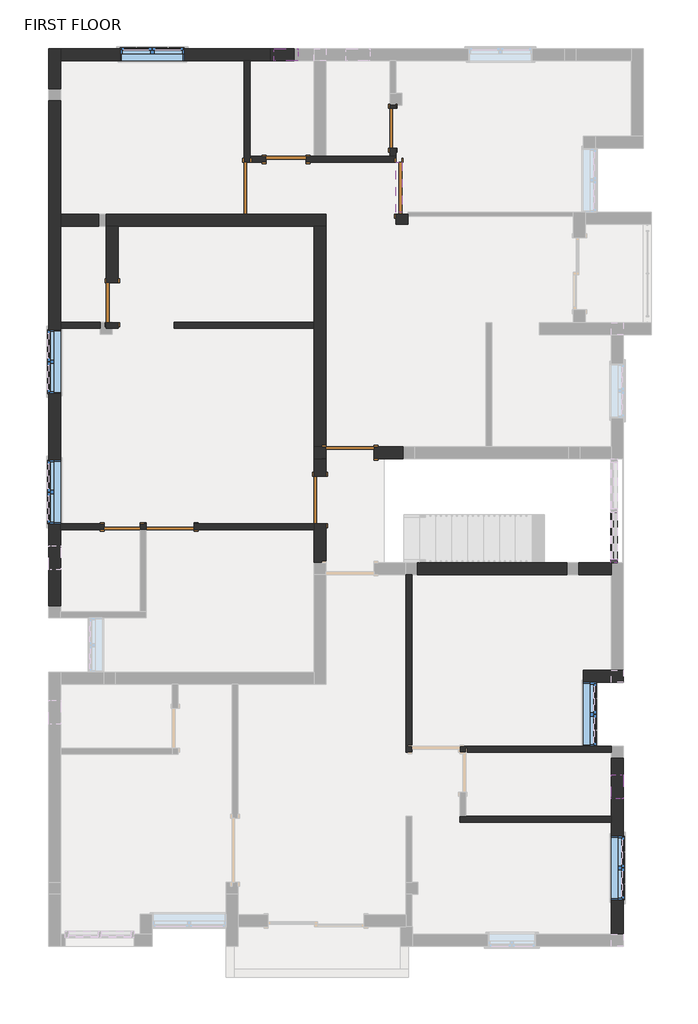
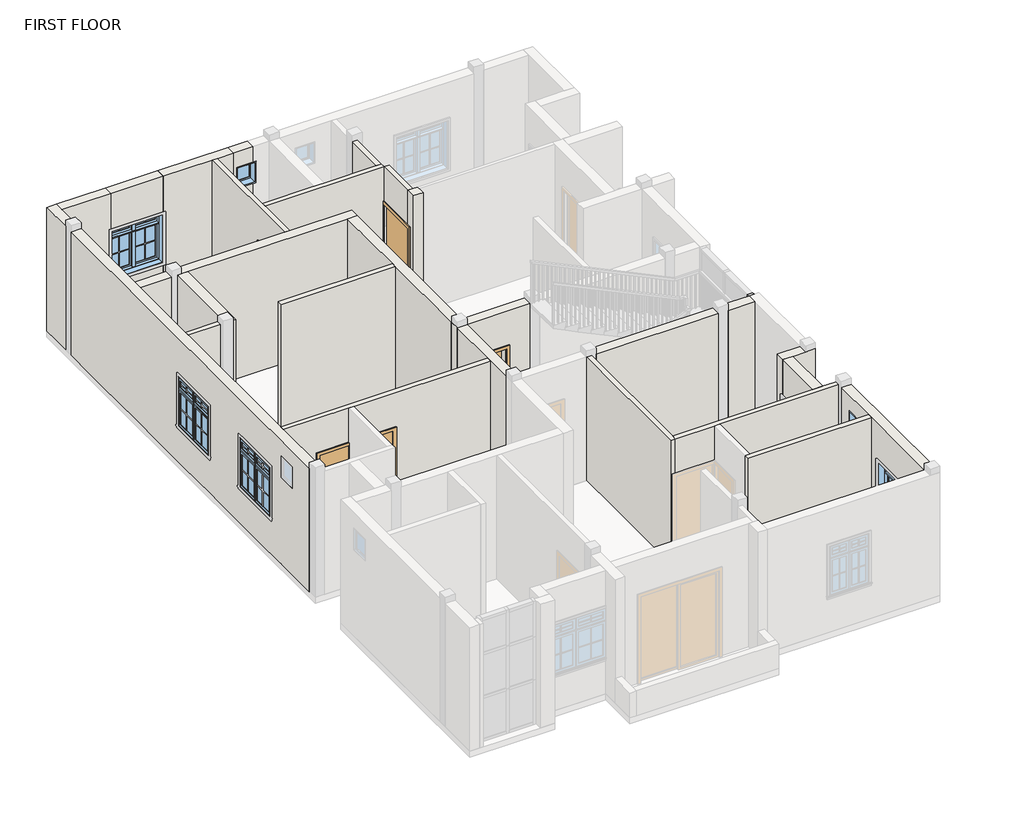
# One storey, part 2 of 6: 29 walls, 9 doors, 7 windows, 3 members.
"""IFC4 building model written with IfcOpenShell, lengths in millimetres."""

from ifc_helpers import new_model, si_unit, frame, origin, place, context, project, spatial, polyline, outline, extrude, faceted_brep, transform, mapped, element, save
from components import door_64f31108, door_78caadf7, door_214872d5, door_bb98abfd, door_43e5c869, door_0217d254, single_flush_3_x7_a90ba1ad, single_flush_3_x7_e5f9f3c4, member_f1f71bde, member_00c01c4d, member_ecafcbb3, window_abb441dd, window_casement_double_awning_double_4_x4_dd9041c6

model = new_model("IFC4")

# Units and contexts
model_context = context("Model", 3, world=origin())
ifc_project = project(units=[si_unit("LENGTHUNIT", "METRE", prefix="MILLI")], contexts=[model_context])

# Site, building, storey
site = spatial("IfcSite", under=ifc_project)
building = spatial("IfcBuilding", under=site)
storey = spatial("IfcBuildingStorey", under=building, Name="FIRST FLOOR", Elevation=3200.4)

# Doors
placement = place(None, origin())
door_shape = door_64f31108(model_context)
element("IfcDoor", 1, ObjectType="Single-Flush : 2'3\"X7'", at=placement, inside=storey, context=model_context, shape_type="MappedRepresentation", body=[
    mapped(door_shape, transform((-5358.7865981, 175.2287587, 3200.4), x_axis=(1.0, 0.0, 0.0), y_axis=(0.0, 1.0, 0.0), z_axis=(0.0, 0.0, 1.0))),
])
door_2_shape = door_78caadf7(model_context)
element("IfcDoor", 2, ObjectType="Single-Flush : 2'6\"X7'", at=placement, inside=storey, context=model_context, shape_type="MappedRepresentation", body=[
    mapped(door_2_shape, transform((-196.2365981, 7776.1787587, 3200.4), x_axis=(0.0, -1.0, 0.0), y_axis=(1.0, 0.0, 0.0), z_axis=(0.0, 0.0, 1.0))),
])
door_3_shape = door_214872d5(model_context)
element("IfcDoor", 3, ObjectType="Single-Flush : 2'6\"X7'", at=placement, inside=storey, context=model_context, shape_type="MappedRepresentation", body=[
    mapped(door_3_shape, transform((-2234.5865981, 7185.6287587, 3200.4), x_axis=(1.0, 0.0, 0.0), y_axis=(0.0, 1.0, 0.0), z_axis=(0.0, 0.0, 1.0))),
])
door_4_shape = door_bb98abfd(model_context)
element("IfcDoor", 4, ObjectType="Single-Flush : 2'6\"X7'", at=placement, inside=storey, context=model_context, shape_type="MappedRepresentation", body=[
    mapped(door_4_shape, transform((-5549.2865981, 4455.1287587, 3200.4), x_axis=(0.0, 1.0, 0.0), y_axis=(-1.0, 0.0, 0.0), z_axis=(0.0, 0.0, 1.0))),
])
door_5_shape = door_43e5c869(model_context)
element("IfcDoor", 5, ObjectType="Single-Flush : 3'3\"X7'", at=placement, inside=storey, context=model_context, shape_type="MappedRepresentation", body=[
    mapped(door_5_shape, transform((-2977.5365981, 6633.1787587, 3200.4), x_axis=(0.0, -1.0, 0.0), y_axis=(1.0, 0.0, 0.0), z_axis=(0.0, 0.0, 1.0))),
])
door_6_shape = door_0217d254(model_context)
element("IfcDoor", 6, ObjectType="Single-Flush : 3'3\"X7'", at=placement, inside=storey, context=model_context, shape_type="MappedRepresentation", body=[
    mapped(door_6_shape, transform((-81.9365981, 6633.1787587, 3200.4), x_axis=(0.0, -1.0, 0.0), y_axis=(1.0, 0.0, 0.0), z_axis=(0.0, 0.0, 1.0))),
])
single_flush_3_x7_shape = single_flush_3_x7_a90ba1ad(model_context)
element("IfcDoor", 7, ObjectType="Single-Flush : 3'X7'", at=placement, inside=storey, context=model_context, shape_type="MappedRepresentation", body=[
    mapped(single_flush_3_x7_shape, transform((-1586.8865981, 689.5787587, 3200.4), x_axis=(0.0, -1.0, 0.0), y_axis=(1.0, 0.0, 0.0), z_axis=(0.0, 0.0, 1.0))),
])
element("IfcDoor", 8, ObjectType="Single-Flush : 3'X7'", at=placement, inside=storey, context=model_context, shape_type="MappedRepresentation", body=[
    mapped(single_flush_3_x7_shape, transform((-1015.3865981, 1591.2787587, 3200.4), x_axis=(-1.0, 0.0, 0.0), y_axis=(0.0, -1.0, 0.0), z_axis=(0.0, 0.0, 1.0))),
])
single_flush_3_x7_2_shape = single_flush_3_x7_e5f9f3c4(model_context)
element("IfcDoor", 9, ObjectType="Single-Flush : 3'X7'", at=placement, inside=storey, context=model_context, shape_type="MappedRepresentation", body=[
    mapped(single_flush_3_x7_2_shape, transform((-4444.3865981, 175.2287587, 3200.4), x_axis=(-1.0, 0.0, 0.0), y_axis=(0.0, -1.0, 0.0), z_axis=(0.0, 0.0, 1.0))),
])

# Members
member_shape = member_f1f71bde(model_context)
element("IfcMember", 10, ObjectType="Rectangular Mullion : 2.5\" x 5\" rectangular", at=placement, inside=storey, context=model_context, shape_type="MappedRepresentation", body=[
    mapped(member_shape, transform((4026.5134019, -440.7212413, 3200.4), x_axis=(0.0, 0.0, -1.0), y_axis=(1.0, 0.0, 0.0), z_axis=(0.0, -1.0, 0.0))),
])
member_2_shape = member_00c01c4d(model_context)
element("IfcMember", 11, ObjectType="Rectangular Mullion : 2.5\" x 5\" rectangular", at=placement, inside=storey, context=model_context, shape_type="MappedRepresentation", body=[
    mapped(member_2_shape, transform((4026.5134019, -504.2212413, 4756.15), x_axis=(0.0, -1.0, 0.0), y_axis=(1.0, 0.0, 0.0), z_axis=(0.0, 0.0, 1.0))),
])
member_3_shape = member_ecafcbb3(model_context)
element("IfcMember", 12, ObjectType="Rectangular Mullion : 2.5\" x 5\" rectangular", at=placement, inside=storey, context=model_context, shape_type="MappedRepresentation", body=[
    mapped(member_3_shape, transform((4026.5134019, -504.2212413, 6248.4), x_axis=(0.0, -1.0, 0.0), y_axis=(1.0, 0.0, 0.0), z_axis=(0.0, 0.0, 1.0))),
])

# Walls
element("IfcWall", 13, ObjectType="4.5\"", at=placement, inside=storey, context=model_context, shape_type="Brep", body=[
    faceted_brep([(-3034.6865981, 6137.8787587, 6248.4), (-3034.6865981, 9071.5787587, 6248.4), (-3034.6865981, 9071.5787587, 3200.4), (-3034.6865981, 7128.4787587, 3200.4), (-3034.6865981, 7128.4787587, 5334.0), (-3034.6865981, 6137.8787587, 5334.0), (-2920.3865981, 9071.5787587, 6248.4), (-2920.3865981, 7242.7787587, 6248.4), (-2920.3865981, 7128.4787587, 6248.4), (-2920.3865981, 6137.8787587, 6248.4), (-2920.3865981, 6137.8787587, 5334.0), (-2920.3865981, 7128.4787587, 5334.0), (-2920.3865981, 7128.4787587, 3200.4), (-2920.3865981, 7242.7787587, 3200.4), (-2920.3865981, 9071.5787587, 3200.4)], [[[0, 1, 2, 3, 4, 5]], [[6, 7, 8, 9, 10, 11, 12, 13, 14]], [[2, 14, 13, 12, 3]], [[1, 0, 9, 8, 7, 6]], [[2, 1, 6, 14]], [[9, 0, 5, 10]], [[4, 11, 10, 5]], [[11, 4, 3, 12]]]),
])
element("IfcWall", 14, ObjectType="4.5\"", at=placement, inside=storey, context=model_context, shape_type="Brep", body=[
    faceted_brep([(-1853.5865981, 7128.4787587, 5334.0), (-1853.5865981, 7128.4787587, 3200.4), (-139.0865981, 7128.4787587, 3200.4), (-139.0865981, 7128.4787587, 6248.4), (-2920.3865981, 7128.4787587, 6248.4), (-2920.3865981, 7128.4787587, 5334.0), (-2920.3865981, 7128.4787587, 3200.4), (-2615.5865981, 7128.4787587, 3200.4), (-2615.5865981, 7128.4787587, 5334.0), (-139.0865981, 7242.7787587, 3200.4), (-253.3865981, 7242.7787587, 3200.4), (-1472.5865981, 7242.7787587, 3200.4), (-1701.1865981, 7242.7787587, 3200.4), (-1853.5865981, 7242.7787587, 3200.4), (-1853.5865981, 7242.7787587, 5334.0), (-2615.5865981, 7242.7787587, 5334.0), (-2615.5865981, 7242.7787587, 3200.4), (-2920.3865981, 7242.7787587, 3200.4), (-2920.3865981, 7242.7787587, 6248.4), (-1701.1865981, 7242.7787587, 6248.4), (-1472.5865981, 7242.7787587, 6248.4), (-253.3865981, 7242.7787587, 6248.4), (-139.0865981, 7242.7787587, 6248.4)], [[[0, 1, 2, 3, 4, 5, 6, 7, 8]], [[9, 10, 11, 12, 13, 14, 15, 16, 17, 18, 19, 20, 21, 22]], [[7, 6, 17, 16]], [[2, 1, 13, 12, 11, 10, 9]], [[4, 3, 22, 21, 20, 19, 18]], [[6, 5, 4, 18, 17]], [[3, 2, 9, 22]], [[14, 13, 1, 0]], [[15, 14, 0, 8]], [[16, 15, 8, 7]]]),
])
element("IfcWall", 15, ObjectType="4.5\"", at=placement, inside=storey, context=model_context, shape_type="SweptSolid", body=[
    extrude(outline(polyline([(7395.1787587, 5334.0), (7395.1787587, 3200.4), (7242.7787587, 3200.4), (7242.7787587, 6248.4), (8214.4921256, 6248.4), (8214.4921256, 3200.4), (8157.1787587, 3200.4), (8157.1787587, 5334.0), (7395.1787587, 5334.0)])), frame((-253.3865981, 0.0, 0.0), z_axis=(1.0, 0.0, 0.0), x_axis=(0.0, 1.0, 0.0)), (0.0, 0.0, 1.0), 114.3),
])
element("IfcWall", 16, ObjectType="4.5\"", at=placement, inside=storey, context=model_context, shape_type="SweptSolid", body=[
    extrude(outline(polyline([(-4368.1865981, 4080.4787587), (-1701.1865981, 4080.4787587), (-1701.1865981, 3966.1787587), (-4368.1865981, 3966.1787587), (-4368.1865981, 4080.4787587)])), frame((0.0, 0.0, 3200.4), z_axis=(0.0, 0.0, 1.0), x_axis=(1.0, 0.0, 0.0)), (0.0, 0.0, 1.0), 3048.0),
])
element("IfcWall", 17, ObjectType="4.5\"", at=placement, inside=storey, context=model_context, shape_type="SweptSolid", body=[
    extrude(outline(polyline([(-5786.6284021, 3966.1787587), (-6539.8865981, 3966.1787587), (-6539.8865981, 4080.4787587), (-5786.6284021, 4080.4787587), (-5786.6284021, 3966.1787587)])), frame((0.0, 0.0, 3200.4), z_axis=(0.0, 0.0, 1.0), x_axis=(1.0, 0.0, 0.0)), (0.0, 0.0, 1.0), 3048.0),
])
element("IfcWall", 18, ObjectType="4.5\"", at=placement, inside=storey, context=model_context, shape_type="Brep", body=[
    faceted_brep([(-5663.5865981, 4080.4787587, 6248.4), (-5558.0284021, 4080.4787587, 6248.4), (-5434.9865981, 4080.4787587, 6248.4), (-5434.9865981, 4080.4787587, 5334.0), (-5558.0284021, 4080.4787587, 5334.0), (-5663.5865981, 4080.4787587, 5334.0), (-5663.5865981, 3966.1787587, 3200.4), (-5558.0284021, 3966.1787587, 3200.4), (-5434.9865981, 3966.1787587, 3200.4), (-5434.9865981, 3966.1787587, 6248.4), (-5558.0284021, 3966.1787587, 6248.4), (-5663.5865981, 3966.1787587, 6248.4), (-5663.5865981, 4074.1287587, 3200.4), (-5558.0284021, 4074.1287587, 3200.4), (-5434.9865981, 4074.1287587, 3200.4), (-5434.9865981, 4074.1287587, 5334.0), (-5558.0284021, 4074.1287587, 5334.0), (-5663.5865981, 4074.1287587, 5334.0)], [[[0, 1, 2, 3, 4, 5]], [[6, 7, 8, 9, 10, 11]], [[8, 7, 6, 12, 13, 14]], [[2, 1, 0, 11, 10, 9]], [[9, 8, 14, 15, 3, 2]], [[15, 16, 17, 5, 4, 3]], [[17, 16, 15, 14, 13, 12]], [[6, 11, 0, 5, 17, 12]]]),
])
element("IfcWall", 19, ObjectType="4.5\"", at=placement, inside=storey, context=model_context, shape_type="Brep", body=[
    faceted_brep([(-4901.5865981, 232.3787587, 3200.4), (-5015.8865981, 232.3787587, 3200.4), (-5015.8865981, 232.3787587, 5334.0), (-5701.6865981, 232.3787587, 5334.0), (-5701.6865981, 232.3787587, 3200.4), (-6539.8865981, 232.3787587, 3200.4), (-6539.8865981, 232.3787587, 4114.8), (-6539.8865981, 232.3787587, 5334.0), (-6539.8865981, 232.3787587, 6248.4), (-1701.1865981, 232.3787587, 6248.4), (-1701.1865981, 232.3787587, 5334.0), (-1701.1865981, 232.3787587, 3200.4), (-3987.1865981, 232.3787587, 3200.4), (-3987.1865981, 232.3787587, 5334.0), (-4901.5865981, 232.3787587, 5334.0), (-5015.8865981, 118.0787587, 5334.0), (-5015.8865981, 118.0787587, 3200.4), (-4901.5865981, 118.0787587, 3200.4), (-4901.5865981, 118.0787587, 5334.0), (-3987.1865981, 118.0787587, 5334.0), (-3987.1865981, 118.0787587, 3200.4), (-1701.1865981, 118.0787587, 3200.4), (-1701.1865981, 118.0787587, 6248.4), (-4901.5865981, 118.0787587, 6248.4), (-5015.8865981, 118.0787587, 6248.4), (-6539.8865981, 118.0787587, 6248.4), (-6539.8865981, 118.0787587, 3200.4), (-5701.6865981, 118.0787587, 3200.4), (-5701.6865981, 118.0787587, 5334.0)], [[[0, 1, 2, 3, 4, 5, 6, 7, 8, 9, 10, 11, 12, 13, 14]], [[15, 16, 17, 18, 19, 20, 21, 22, 23, 24, 25, 26, 27, 28]], [[12, 11, 21, 20]], [[27, 26, 5, 4]], [[17, 16, 1, 0]], [[9, 8, 25, 24, 23, 22]], [[8, 7, 6, 5, 26, 25]], [[11, 10, 9, 22, 21]], [[18, 17, 0, 14]], [[19, 18, 14, 13]], [[20, 19, 13, 12]], [[2, 1, 16, 15]], [[3, 2, 15, 28]], [[4, 3, 28, 27]]]),
])
element("IfcWall", 20, ObjectType="4.5\"", at=placement, inside=storey, context=model_context, shape_type="Brep", body=[
    faceted_brep([(51.4134019, -732.8212413, 3200.4), (51.4134019, -4123.7212413, 3200.4), (51.4134019, -4123.7212413, 6248.4), (51.4134019, -732.8212413, 6248.4), (165.7134019, -732.8212413, 3200.4), (165.7134019, -732.8212413, 6248.4), (165.7134019, -4009.4212413, 6248.4), (165.7134019, -4123.7212413, 6248.4), (165.7134019, -4123.7212413, 5334.0), (165.7134019, -4123.7212413, 3200.4)], [[[0, 1, 2, 3]], [[4, 5, 6, 7, 8, 9]], [[1, 0, 4, 9]], [[3, 2, 7, 6, 5]], [[0, 3, 5, 4]], [[2, 1, 9, 8, 7]]]),
])
element("IfcWall", 21, ObjectType="4.5\"", at=placement, inside=storey, context=model_context, shape_type="Brep", body=[
    faceted_brep([(3975.7134019, -4123.7212413, 3200.4), (3975.7134019, -4123.7212413, 6248.4), (1194.4134019, -4123.7212413, 6248.4), (1080.1134019, -4123.7212413, 6248.4), (165.7134019, -4123.7212413, 6248.4), (165.7134019, -4123.7212413, 5334.0), (1080.1134019, -4123.7212413, 5334.0), (1080.1134019, -4123.7212413, 3200.4), (1194.4134019, -4123.7212413, 3200.4), (3975.7134019, -4009.4212413, 6248.4), (3975.7134019, -4009.4212413, 3200.4), (3670.9134019, -4009.4212413, 3200.4), (3442.3134019, -4009.4212413, 3200.4), (1080.1134019, -4009.4212413, 3200.4), (1080.1134019, -4009.4212413, 5334.0), (165.7134019, -4009.4212413, 5334.0), (165.7134019, -4009.4212413, 6248.4), (3442.3134019, -4009.4212413, 6248.4), (3670.9134019, -4009.4212413, 6248.4)], [[[0, 1, 2, 3, 4, 5, 6, 7, 8]], [[9, 10, 11, 12, 13, 14, 15, 16, 17, 18]], [[10, 0, 8, 7, 13, 12, 11]], [[1, 0, 10, 9]], [[4, 3, 2, 1, 9, 18, 17, 16]], [[4, 16, 15, 5]], [[14, 6, 5, 15]], [[6, 14, 13, 7]]]),
])
element("IfcWall", 22, ObjectType="4.5\"", at=placement, inside=storey, context=model_context, shape_type="Brep", body=[
    faceted_brep([(3975.7134019, -5342.9212413, 3200.4), (1194.4134019, -5342.9212413, 3200.4), (1080.1134019, -5342.9212413, 3200.4), (1080.1134019, -5342.9212413, 6248.4), (1194.4134019, -5342.9212413, 6248.4), (3975.7134019, -5342.9212413, 6248.4), (3975.7134019, -5457.2212413, 3200.4), (3975.7134019, -5457.2212413, 6248.4), (1080.1134019, -5457.2212413, 6248.4), (1080.1134019, -5457.2212413, 3200.4)], [[[0, 1, 2, 3, 4, 5]], [[6, 7, 8, 9]], [[2, 1, 0, 6, 9]], [[5, 4, 3, 8, 7]], [[0, 5, 7, 6]], [[3, 2, 9, 8]]]),
])
element("IfcWall", 23, ObjectType="4.5\"", at=placement, inside=storey, context=model_context, shape_type="SweptSolid", body=[
    extrude(outline(polyline([(-139.0865981, 6175.9787587), (-139.0865981, 7128.4787587), (-24.7865981, 7128.4787587), (-24.7865981, 6175.9787587), (-139.0865981, 6175.9787587)])), frame((0.0, 0.0, 5334.0), z_axis=(0.0, 0.0, 1.0), x_axis=(1.0, 0.0, 0.0)), (0.0, 0.0, 1.0), 914.4),
])
element("IfcWall", 24, ObjectType="9\"", at=placement, inside=storey, context=model_context, shape_type="Brep", body=[
    faceted_brep([(-6768.4865981, 9300.1787587, 3200.4), (-6768.4865981, 8531.2343988, 3200.4), (-6768.4865981, 8531.2343988, 6248.4), (-6768.4865981, 9300.1787587, 6248.4), (-6539.8865981, 9300.1787587, 3200.4), (-6539.8865981, 9300.1787587, 6248.4), (-6539.8865981, 9071.5787587, 6248.4), (-6539.8865981, 8531.2343988, 6248.4), (-6539.8865981, 8531.2343988, 3200.4), (-6539.8865981, 9071.5787587, 3200.4)], [[[0, 1, 2, 3]], [[4, 5, 6, 7, 8, 9]], [[1, 0, 4, 9, 8]], [[2, 1, 8, 7]], [[3, 2, 7, 6, 5]], [[0, 3, 5, 4]]]),
])
element("IfcWall", 25, ObjectType="9\"", at=placement, inside=storey, context=model_context, shape_type="Brep", body=[
    faceted_brep([(-6768.4865981, 8302.6343988, 3200.4), (-6768.4865981, -1329.7212413, 3200.4), (-6768.4865981, -1329.7212413, 6248.4), (-6768.4865981, 8302.6343988, 6248.4), (-6768.4865981, 1451.5787587, 5334.0), (-6768.4865981, 232.3787587, 5334.0), (-6768.4865981, 232.3787587, 4114.8), (-6768.4865981, 1451.5787587, 4114.8), (-6768.4865981, 3937.3572861, 5334.0), (-6768.4865981, 2718.1572861, 5334.0), (-6768.4865981, 2718.1572861, 4114.8), (-6768.4865981, 3937.3572861, 4114.8), (-6768.4865981, -186.7212413, 5867.4), (-6768.4865981, -643.9212413, 5867.4), (-6768.4865981, -643.9212413, 5334.0), (-6768.4865981, -186.7212413, 5334.0), (-6539.8865981, 8302.6343988, 3200.4), (-6539.8865981, 8302.6343988, 6248.4), (-6539.8865981, 6137.8787587, 6248.4), (-6539.8865981, 5909.2787587, 6248.4), (-6539.8865981, 4080.4787587, 6248.4), (-6539.8865981, 3966.1787587, 6248.4), (-6539.8865981, 232.3787587, 6248.4), (-6539.8865981, 118.0787587, 6248.4), (-6539.8865981, -1329.7212413, 6248.4), (-6539.8865981, -1329.7212413, 3200.4), (-6539.8865981, 118.0787587, 3200.4), (-6539.8865981, 232.3787587, 3200.4), (-6539.8865981, 3966.1787587, 3200.4), (-6539.8865981, 4080.4787587, 3200.4), (-6539.8865981, 5909.2787587, 3200.4), (-6539.8865981, 6137.8787587, 3200.4), (-6539.8865981, 1451.5787587, 5334.0), (-6539.8865981, 1451.5787587, 4114.8), (-6539.8865981, 232.3787587, 4114.8), (-6539.8865981, 232.3787587, 5334.0), (-6539.8865981, 3937.3572861, 5334.0), (-6539.8865981, 3937.3572861, 4114.8), (-6539.8865981, 2718.1572861, 4114.8), (-6539.8865981, 2718.1572861, 5334.0), (-6539.8865981, -186.7212413, 5867.4), (-6539.8865981, -186.7212413, 5334.0), (-6539.8865981, -643.9212413, 5334.0), (-6539.8865981, -643.9212413, 5867.4)], [[[0, 1, 2, 3], [4, 5, 6, 7], [8, 9, 10, 11], [12, 13, 14, 15]], [[16, 17, 18, 19, 20, 21, 22, 23, 24, 25, 26, 27, 28, 29, 30, 31], [32, 33, 34, 35], [36, 37, 38, 39], [40, 41, 42, 43]], [[1, 0, 16, 31, 30, 29, 28, 27, 26, 25]], [[2, 1, 25, 24]], [[3, 2, 24, 23, 22, 21, 20, 19, 18, 17]], [[0, 3, 17, 16]], [[33, 32, 4, 7]], [[34, 33, 7, 6]], [[35, 34, 6, 5]], [[32, 35, 5, 4]], [[37, 36, 8, 11]], [[38, 37, 11, 10]], [[39, 38, 10, 9]], [[36, 39, 9, 8]], [[41, 40, 12, 15]], [[42, 41, 15, 14]], [[43, 42, 14, 13]], [[40, 43, 13, 12]]]),
])
element("IfcWall", 26, ObjectType="9\"", at=placement, inside=storey, context=model_context, shape_type="Brep", body=[
    faceted_brep([(4204.3134019, -7590.8212413, 3200.4), (4204.3134019, -4238.0212413, 3200.4), (4204.3134019, -4238.0212413, 6248.4), (4204.3134019, -7590.8212413, 6248.4), (4204.3134019, -6938.5380734, 5334.0), (4204.3134019, -5719.3380734, 5334.0), (4204.3134019, -5719.3380734, 4114.8), (4204.3134019, -6938.5380734, 4114.8), (4204.3134019, -5004.2995612, 5867.4), (4204.3134019, -4547.0995612, 5867.4), (4204.3134019, -4547.0995612, 5334.0), (4204.3134019, -5004.2995612, 5334.0), (3975.7134019, -7590.8212413, 3200.4), (3975.7134019, -7590.8212413, 6248.4), (3975.7134019, -5457.2212413, 6248.4), (3975.7134019, -5342.9212413, 6248.4), (3975.7134019, -4238.0212413, 6248.4), (3975.7134019, -4238.0212413, 3200.4), (3975.7134019, -5342.9212413, 3200.4), (3975.7134019, -5457.2212413, 3200.4), (3975.7134019, -6938.5380734, 5334.0), (3975.7134019, -6938.5380734, 4114.8), (3975.7134019, -5719.3380734, 4114.8), (3975.7134019, -5719.3380734, 5334.0), (3975.7134019, -5004.2995612, 5867.4), (3975.7134019, -5004.2995612, 5334.0), (3975.7134019, -4547.0995612, 5334.0), (3975.7134019, -4547.0995612, 5867.4)], [[[0, 1, 2, 3], [4, 5, 6, 7], [8, 9, 10, 11]], [[12, 13, 14, 15, 16, 17, 18, 19], [20, 21, 22, 23], [24, 25, 26, 27]], [[1, 0, 12, 19, 18, 17]], [[2, 1, 17, 16]], [[3, 2, 16, 15, 14, 13]], [[0, 3, 13, 12]], [[21, 20, 4, 7]], [[22, 21, 7, 6]], [[23, 22, 6, 5]], [[20, 23, 5, 4]], [[25, 24, 8, 11]], [[26, 25, 11, 10]], [[27, 26, 10, 9]], [[24, 27, 9, 8]]]),
])
element("IfcWall", 27, ObjectType="9\"", at=placement, inside=storey, context=model_context, shape_type="SweptSolid", body=[
    extrude(outline(polyline([(3670.9134019, -2790.2212413), (3670.9134019, -4009.4212413), (3442.3134019, -4009.4212413), (3442.3134019, -2790.2212413), (3670.9134019, -2790.2212413)])), frame((0.0, 0.0, 3200.4), z_axis=(0.0, 0.0, 1.0), x_axis=(1.0, 0.0, 0.0)), (0.0, 0.0, 1.0), 914.4),
    extrude(outline(polyline([(3670.9134019, -2790.2212413), (3670.9134019, -4009.4212413), (3442.3134019, -4009.4212413), (3442.3134019, -2790.2212413), (3670.9134019, -2790.2212413)])), frame((0.0, 0.0, 5334.0), z_axis=(0.0, 0.0, 1.0), x_axis=(1.0, 0.0, 0.0)), (0.0, 0.0, 1.0), 914.4),
])
element("IfcWall", 28, ObjectType="9\"", at=placement, inside=storey, context=model_context, shape_type="Brep", body=[
    faceted_brep([(3442.3134019, -2790.2212413, 3200.4), (3670.9134019, -2790.2212413, 3200.4), (4204.3134019, -2790.2212413, 3200.4), (4204.3134019, -2790.2212413, 6248.4), (3975.7134019, -2790.2212413, 6248.4), (3670.9134019, -2790.2212413, 6248.4), (3442.3134019, -2790.2212413, 6248.4), (3442.3134019, -2790.2212413, 5334.0), (3442.3134019, -2790.2212413, 4114.8), (3442.3134019, -2561.6212413, 3200.4), (3442.3134019, -2561.6212413, 6248.4), (3975.7134019, -2561.6212413, 6248.4), (4204.3134019, -2561.6212413, 6248.4), (4204.3134019, -2561.6212413, 3200.4), (3975.7134019, -2561.6212413, 3200.4)], [[[0, 1, 2, 3, 4, 5, 6, 7, 8]], [[9, 10, 11, 12, 13, 14]], [[2, 1, 0, 9, 14, 13]], [[6, 5, 4, 3, 12, 11, 10]], [[0, 8, 7, 6, 10, 9]], [[3, 2, 13, 12]]]),
])
element("IfcWall", 29, ObjectType="9\"", at=placement, inside=storey, context=model_context, shape_type="SweptSolid", body=[
    extrude(outline(polyline([(3352.7127672, -504.2212413), (3975.7134019, -504.2212413), (3975.7134019, -732.8212413), (3352.7127672, -732.8212413), (3352.7127672, -504.2212413)])), frame((0.0, 0.0, 3200.4), z_axis=(0.0, 0.0, 1.0), x_axis=(1.0, 0.0, 0.0)), (0.0, 0.0, 1.0), 3048.0),
])
element("IfcWall", 30, ObjectType="9\"", at=placement, inside=storey, context=model_context, shape_type="SweptSolid", body=[
    extrude(outline(polyline([(269.7035962, -504.2212413), (3124.1127672, -504.2212413), (3124.1127672, -732.8212413), (269.7035962, -732.8212413), (269.7035962, -504.2212413)])), frame((0.0, 0.0, 3200.4), z_axis=(0.0, 0.0, 1.0), x_axis=(1.0, 0.0, 0.0)), (0.0, 0.0, 1.0), 3048.0),
])
element("IfcWall", 31, ObjectType="9\"", at=placement, inside=storey, context=model_context, shape_type="Brep", body=[
    faceted_brep([(-1472.5865981, 1705.5787587, 5334.0), (-1472.5865981, 1705.5787587, 3200.4), (-1701.1865981, 1705.5787587, 3200.4), (-1701.1865981, 1705.5787587, 6248.4), (-1472.5865981, 1705.5787587, 6248.4), (0.651657, 1705.5787587, 6248.4), (0.651657, 1705.5787587, 3200.4), (-558.1865981, 1705.5787587, 3200.4), (-558.1865981, 1705.5787587, 5334.0), (-1701.1865981, 1476.9787587, 3200.4), (-1472.5865981, 1476.9787587, 3200.4), (-1472.5865981, 1476.9787587, 5334.0), (-558.1865981, 1476.9787587, 5334.0), (-558.1865981, 1476.9787587, 3200.4), (0.651657, 1476.9787587, 3200.4), (0.651657, 1476.9787587, 6248.4), (-1472.5865981, 1476.9787587, 6248.4), (-1701.1865981, 1476.9787587, 6248.4), (-1701.1865981, 1693.0966521, 6248.4)], [[[0, 1, 2, 3, 4, 5, 6, 7, 8]], [[9, 10, 11, 12, 13, 14, 15, 16, 17]], [[7, 6, 14, 13]], [[2, 1, 10, 9]], [[5, 4, 3, 18, 17, 16, 15]], [[6, 5, 15, 14]], [[3, 2, 9, 17, 18]], [[11, 10, 1, 0]], [[12, 11, 0, 8]], [[13, 12, 8, 7]]]),
])
element("IfcWall", 32, ObjectType="9\"", at=placement, inside=storey, context=model_context, shape_type="Brep", body=[
    faceted_brep([(-2539.3865981, 9300.1787587, 3200.4), (-4177.6865981, 9300.1787587, 3200.4), (-4177.6865981, 9300.1787587, 4114.8), (-4177.6865981, 9300.1787587, 5334.0), (-4177.6865981, 9300.1787587, 6248.4), (-2539.3865981, 9300.1787587, 6248.4), (-2539.3865981, 9071.5787587, 3200.4), (-2539.3865981, 9071.5787587, 6248.4), (-2920.3865981, 9071.5787587, 6248.4), (-3034.6865981, 9071.5787587, 6248.4), (-4177.6865981, 9071.5787587, 6248.4), (-4177.6865981, 9071.5787587, 5334.0), (-4177.6865981, 9071.5787587, 4114.8), (-4177.6865981, 9071.5787587, 3200.4), (-3034.6865981, 9071.5787587, 3200.4), (-2920.3865981, 9071.5787587, 3200.4)], [[[0, 1, 2, 3, 4, 5]], [[6, 7, 8, 9, 10, 11, 12, 13, 14, 15]], [[1, 0, 6, 15, 14, 13]], [[4, 3, 2, 1, 13, 12, 11, 10]], [[5, 4, 10, 9, 8, 7]], [[0, 5, 7, 6]]]),
])
element("IfcWall", 33, ObjectType="9\"", at=placement, inside=storey, context=model_context, shape_type="Brep", body=[
    faceted_brep([(-5396.8865981, 9300.1787587, 3200.4), (-6539.8865981, 9300.1787587, 3200.4), (-6539.8865981, 9300.1787587, 6248.4), (-5396.8865981, 9300.1787587, 6248.4), (-5396.8865981, 9300.1787587, 5334.0), (-5396.8865981, 9300.1787587, 4114.8), (-5396.8865981, 9071.5787587, 3200.4), (-5396.8865981, 9071.5787587, 4114.8), (-5396.8865981, 9071.5787587, 5334.0), (-5396.8865981, 9071.5787587, 6248.4), (-6539.8865981, 9071.5787587, 6248.4), (-6539.8865981, 9071.5787587, 3200.4)], [[[0, 1, 2, 3, 4, 5]], [[6, 7, 8, 9, 10, 11]], [[1, 0, 6, 11]], [[3, 2, 10, 9]], [[0, 5, 4, 3, 9, 8, 7, 6]], [[2, 1, 11, 10]]]),
])
element("IfcWall", 34, ObjectType="9\"", at=placement, inside=storey, context=model_context, shape_type="SweptSolid", body=[
    extrude(outline(polyline([(-5807.056564, 5909.2787587), (-6539.8865981, 5909.2787587), (-6539.8865981, 6137.8787587), (-5807.056564, 6137.8787587), (-5807.056564, 5909.2787587)])), frame((0.0, 0.0, 3200.4), z_axis=(0.0, 0.0, 1.0), x_axis=(1.0, 0.0, 0.0)), (0.0, 0.0, 1.0), 3048.0),
])
element("IfcWall", 35, ObjectType="9\"", at=placement, inside=storey, context=model_context, shape_type="Brep", body=[
    faceted_brep([(-5663.5865981, 5909.2787587, 3200.4), (-5434.9865981, 5909.2787587, 3200.4), (-1701.1865981, 5909.2787587, 3200.4), (-1472.5865981, 5909.2787587, 3200.4), (-1472.5865981, 5909.2787587, 6248.4), (-1701.1865981, 5909.2787587, 6248.4), (-5434.9865981, 5909.2787587, 6248.4), (-5578.456564, 5909.2787587, 6248.4), (-5663.5865981, 5909.2787587, 6248.4), (-5663.5865981, 6137.8787587, 3200.4), (-5663.5865981, 6137.8787587, 6248.4), (-5578.456564, 6137.8787587, 6248.4), (-3034.6865981, 6137.8787587, 6248.4), (-2920.3865981, 6137.8787587, 6248.4), (-1472.5865981, 6137.8787587, 6248.4), (-1472.5865981, 6137.8787587, 3200.4)], [[[0, 1, 2, 3, 4, 5, 6, 7, 8]], [[9, 10, 11, 12, 13, 14, 15]], [[3, 2, 1, 0, 9, 15]], [[8, 7, 6, 5, 4, 14, 13, 12, 11, 10]], [[4, 3, 15, 14]], [[0, 8, 10, 9]]]),
])
element("IfcWall", 36, ObjectType="9\"", at=placement, inside=storey, context=model_context, shape_type="Brep", body=[
    faceted_brep([(-1701.1865981, 5909.2787587, 3200.4), (-1701.1865981, 4080.4787587, 3200.4), (-1701.1865981, 3966.1787587, 3200.4), (-1701.1865981, 1705.5787587, 3200.4), (-1701.1865981, 1705.5787587, 6248.4), (-1701.1865981, 3966.1787587, 6248.4), (-1701.1865981, 4080.4787587, 6248.4), (-1701.1865981, 5909.2787587, 6248.4), (-1472.5865981, 5909.2787587, 3200.4), (-1472.5865981, 5909.2787587, 6248.4), (-1472.5865981, 1705.5787587, 6248.4), (-1472.5865981, 1705.5787587, 5334.0), (-1472.5865981, 1705.5787587, 3200.4)], [[[0, 1, 2, 3, 4, 5, 6, 7]], [[8, 9, 10, 11, 12]], [[3, 2, 1, 0, 8, 12]], [[7, 6, 5, 4, 10, 9]], [[0, 7, 9, 8]], [[4, 3, 12, 11, 10]]]),
])
element("IfcWall", 37, ObjectType="9\"", at=placement, inside=storey, context=model_context, shape_type="Brep", body=[
    faceted_brep([(-1701.1865981, 232.3787587, 5334.0), (-1701.1865981, 232.3787587, 3200.4), (-1701.1865981, 118.0787587, 3200.4), (-1701.1865981, -504.2212413, 3200.4), (-1701.1865981, -504.2212413, 6248.4), (-1701.1865981, 118.0787587, 6248.4), (-1701.1865981, 232.3787587, 6248.4), (-1701.1865981, 1464.4966521, 6248.4), (-1701.1865981, 1464.4966521, 3200.4), (-1701.1865981, 1146.7787587, 3200.4), (-1701.1865981, 1146.7787587, 5334.0), (-1472.5865981, -504.2212413, 3200.4), (-1472.5865981, 232.3787587, 3200.4), (-1472.5865981, 232.3787587, 5334.0), (-1472.5865981, 1146.7787587, 5334.0), (-1472.5865981, 1146.7787587, 3200.4), (-1472.5865981, 1464.4966521, 3200.4), (-1472.5865981, 1464.4966521, 6248.4), (-1472.5865981, -504.2212413, 6248.4), (-1472.5865981, -504.2212413, 5334.0)], [[[0, 1, 2, 3, 4, 5, 6, 7, 8, 9, 10]], [[11, 12, 13, 14, 15, 16, 17, 18, 19]], [[9, 8, 16, 15]], [[3, 2, 1, 12, 11]], [[7, 6, 5, 4, 18, 17]], [[8, 7, 17, 16]], [[4, 3, 11, 19, 18]], [[13, 12, 1, 0]], [[14, 13, 0, 10]], [[15, 14, 10, 9]]]),
])
element("IfcWall", 38, ObjectType="9\"", at=placement, inside=storey, context=model_context, shape_type="SweptSolid", body=[
    extrude(outline(polyline([(4080.4787587, 6248.4), (5909.2787587, 6248.4), (5909.2787587, 3200.4), (4836.1287587, 3200.4), (4836.1287587, 5334.0), (4080.4787587, 5334.0), (4080.4787587, 6248.4)])), frame((-5663.5865981, 0.0, 0.0), z_axis=(1.0, 0.0, 0.0), x_axis=(0.0, 1.0, 0.0)), (0.0, 0.0, 1.0), 228.6),
])
element("IfcWall", 39, ObjectType="9\"", at=placement, inside=storey, context=model_context, shape_type="SweptSolid", body=[
    extrude(outline(polyline([(-4177.6865981, 9071.5787587), (-5396.8865981, 9071.5787587), (-5396.8865981, 9300.1787587), (-4177.6865981, 9300.1787587), (-4177.6865981, 9071.5787587)])), frame((0.0, 0.0, 3200.4), z_axis=(0.0, 0.0, 1.0), x_axis=(1.0, 0.0, 0.0)), (0.0, 0.0, 1.0), 914.4),
    extrude(outline(polyline([(-4177.6865981, 9071.5787587), (-5396.8865981, 9071.5787587), (-5396.8865981, 9300.1787587), (-4177.6865981, 9300.1787587), (-4177.6865981, 9071.5787587)])), frame((0.0, 0.0, 5334.0), z_axis=(0.0, 0.0, 1.0), x_axis=(1.0, 0.0, 0.0)), (0.0, 0.0, 1.0), 914.4),
])
element("IfcWall", 40, ObjectType="9\"", at=placement, inside=storey, context=model_context, shape_type="SweptSolid", body=[
    extrude(outline(polyline([(3200.4, -2539.3865981), (3200.4, -2082.1865981), (5334.0, -2082.1865981), (5334.0, -2463.1865981), (5867.4, -2463.1865981), (5867.4, -2082.1865981), (6248.4, -2082.1865981), (6248.4, -2539.3865981), (3200.4, -2539.3865981)])), frame((0.0, 9071.5787587, 0.0), z_axis=(0.0, 1.0, 0.0), x_axis=(0.0, 0.0, 1.0)), (0.0, 0.0, 1.0), 228.6),
])
element("IfcWall", 41, ObjectType="9\"", at=placement, inside=storey, context=model_context, shape_type="Brep", body=[
    faceted_brep([(-139.0865981, 5947.3787587, 3200.4), (-139.0865981, 5947.3787587, 6248.4), (-139.0865981, 6175.9787587, 6248.4), (-139.0865981, 6175.9787587, 5334.0), (-139.0865981, 6137.8787587, 5334.0), (-139.0865981, 6137.8787587, 3200.4), (89.5134019, 5947.3787587, 6248.4), (89.5134019, 5947.3787587, 3200.4), (89.5134019, 6099.7787587, 3200.4), (89.5134019, 6137.8787587, 3200.4), (89.5134019, 6137.8787587, 5334.0), (89.5134019, 6175.9787587, 5334.0), (89.5134019, 6175.9787587, 6248.4), (89.5134019, 6099.7787587, 6248.4), (-24.7865981, 6175.9787587, 6248.4), (-24.7865981, 6175.9787587, 5334.0)], [[[0, 1, 2, 3, 4, 5]], [[6, 7, 8, 9, 10, 11, 12, 13]], [[7, 0, 5, 9, 8]], [[1, 0, 7, 6]], [[2, 1, 6, 13, 12, 14]], [[2, 14, 12, 11, 15, 3]], [[4, 10, 9, 5]], [[10, 4, 3, 15, 11]]]),
])

# Windows
window_shape = window_abb441dd(model_context)
element("IfcWindow", 42, ObjectType="Fixed : 1'6\"X1'9\"", at=placement, inside=storey, context=model_context, shape_type="MappedRepresentation", body=[
    mapped(window_shape, transform((-2196.4865981, 9185.8787587, 3200.4), x_axis=(1.0, 0.0, 0.0), y_axis=(0.0, 1.0, 0.0), z_axis=(0.0, 0.0, 1.0))),
])
element("IfcWindow", 43, ObjectType="Fixed : 1'6\"X1'9\"", at=placement, inside=storey, context=model_context, shape_type="MappedRepresentation", body=[
    mapped(window_shape, transform((4090.0134019, -4813.7995612, 3200.4), x_axis=(0.0, -1.0, 0.0), y_axis=(1.0, 0.0, 0.0), z_axis=(0.0, 0.0, 1.0))),
])
window_casement_double_awning_double_4_x4_shape = window_casement_double_awning_double_4_x4_dd9041c6(model_context)
element("IfcWindow", 44, ObjectType="Window-Casement-Double-Awning-Double : 4'X4'", at=placement, inside=storey, context=model_context, shape_type="MappedRepresentation", body=[
    mapped(window_casement_double_awning_double_4_x4_shape, transform((-4787.2865981, 9185.8787587, 3200.4), x_axis=(1.0, 0.0, 0.0), y_axis=(0.0, 1.0, 0.0), z_axis=(0.0, 0.0, 1.0))),
])
element("IfcWindow", 45, ObjectType="Window-Casement-Double-Awning-Double : 4'X4'", at=placement, inside=storey, context=model_context, shape_type="MappedRepresentation", body=[
    mapped(window_casement_double_awning_double_4_x4_shape, transform((3556.6134019, -3399.8212413, 3200.4), x_axis=(0.0, -1.0, 0.0), y_axis=(1.0, 0.0, 0.0), z_axis=(0.0, 0.0, 1.0))),
])
element("IfcWindow", 46, ObjectType="Window-Casement-Double-Awning-Double : 4'X4'", at=placement, inside=storey, context=model_context, shape_type="MappedRepresentation", body=[
    mapped(window_casement_double_awning_double_4_x4_shape, transform((4090.0134019, -6328.9380734, 3200.4), x_axis=(0.0, -1.0, 0.0), y_axis=(1.0, 0.0, 0.0), z_axis=(0.0, 0.0, 1.0))),
])
element("IfcWindow", 47, ObjectType="Window-Casement-Double-Awning-Double : 4'X4'", at=placement, inside=storey, context=model_context, shape_type="MappedRepresentation", body=[
    mapped(window_casement_double_awning_double_4_x4_shape, transform((-6654.1865981, 841.9787587, 3200.4), x_axis=(0.0, 1.0, 0.0), y_axis=(-1.0, 0.0, 0.0), z_axis=(0.0, 0.0, 1.0))),
])
element("IfcWindow", 48, ObjectType="Window-Casement-Double-Awning-Double : 4'X4'", at=placement, inside=storey, context=model_context, shape_type="MappedRepresentation", body=[
    mapped(window_casement_double_awning_double_4_x4_shape, transform((-6654.1865981, 3327.7572861, 3200.4), x_axis=(0.0, 1.0, 0.0), y_axis=(-1.0, 0.0, 0.0), z_axis=(0.0, 0.0, 1.0))),
])

save(model, "model.ifc")

# Revit data of these elements
# Type "Single-Flush : 2'3\"X7'"
#   Type Mark = "10"
#   Construction Type Id = "MDOOR"
#   Assembly Code = "C1020"
#   Analytic Construction = "Metal"
#   Thickness = 0' - 2"
#   Heat Transfer Coefficient (U) = 0.651978 BTU/(h·ft²·°F)
#   Height = 7' - 0"
#   Trim Projection Ext = 0' - 1"
#   Trim Projection Int = 0' - 1"
#   Trim Width = 0' - 3"
#   Width = 2' - 3"
#   Define Thermal Properties by = 1
#   Door Material = Door - Panel
#   Frame Material = Door - Frame
#   Visual Light Transmittance = 0
#   Solar Heat Gain Coefficient = 0
#   Function = (empty or 0)
#   Wall Closure = (empty or 0)
# Type "Single-Flush : 2'6\"X7'"
#   Type Mark = "9"
#   Construction Type Id = "MDOOR"
#   Assembly Code = "C1020"
#   Analytic Construction = "Metal"
#   Thickness = 0' - 2"
#   Heat Transfer Coefficient (U) = 0.651978 BTU/(h·ft²·°F)
#   Height = 7' - 0"
#   Trim Projection Ext = 0' - 1"
#   Trim Projection Int = 0' - 1"
#   Trim Width = 0' - 3"
#   Width = 2' - 6"
#   Define Thermal Properties by = 1
#   Door Material = Door - Panel
#   Frame Material = Door - Frame
#   Visual Light Transmittance = 0
#   Solar Heat Gain Coefficient = 0
#   Function = (empty or 0)
#   Wall Closure = (empty or 0)
# Type "Single-Flush : 3'3\"X7'"
#   Type Mark = "11"
#   Construction Type Id = "MDOOR"
#   Assembly Code = "C1020"
#   Analytic Construction = "Metal"
#   Thickness = 0' - 2"
#   Heat Transfer Coefficient (U) = 0.651978 BTU/(h·ft²·°F)
#   Height = 7' - 0"
#   Trim Projection Ext = 0' - 1"
#   Trim Projection Int = 0' - 1"
#   Trim Width = 0' - 3"
#   Width = 3' - 3"
#   Define Thermal Properties by = 1
#   Door Material = Door - Panel
#   Frame Material = Door - Frame
#   Visual Light Transmittance = 0
#   Solar Heat Gain Coefficient = 0
#   Function = (empty or 0)
#   Wall Closure = (empty or 0)
# Type "Single-Flush : 3'X7'"
#   Type Mark = "8"
#   Construction Type Id = "MDOOR"
#   Assembly Code = "C1020"
#   Analytic Construction = "Metal"
#   Thickness = 0' - 2"
#   Heat Transfer Coefficient (U) = 0.651978 BTU/(h·ft²·°F)
#   Height = 7' - 0"
#   Trim Projection Ext = 0' - 1"
#   Trim Projection Int = 0' - 1"
#   Trim Width = 0' - 3"
#   Width = 3' - 0"
#   Define Thermal Properties by = 1
#   Door Material = Door - Panel
#   Frame Material = Door - Frame
#   Visual Light Transmittance = 0
#   Solar Heat Gain Coefficient = 0
#   Function = (empty or 0)
#   Wall Closure = (empty or 0)
# Type "Rectangular Mullion : 2.5\" x 5\" rectangular"
#   built-in parameter 1007304 = 0.416667 (stored number, unit not read)
#   built-in parameter 1007301 = 0.104167 (stored number, unit not read)
#   built-in parameter 1007300 = 0.104167 (stored number, unit not read)
# Type "4.5\""
#   Assembly Code = "B2010"
#   Layers, outside or top first: 0' - 4 1/2" no material (function 1)
# Type "9\""
#   Assembly Code = "B2010"
#   Layers, outside or top first: 0' - 9" "wall" (function 1)
# Type "Fixed : 1'6\"X1'9\""
#   Type Mark = "24"
#   Construction Type Id = "GSP4R"
#   Assembly Code = "B2020100"
#   Analytic Construction = "1/8 in Pilkington single glazing"
#   Visual Light Transmittance = 0.9
#   Solar Heat Gain Coefficient = 0.78
#   Heat Transfer Coefficient (U) = 0.6496 BTU/(h·ft²·°F)
#   Height = 1' - 9"
#   Default Sill Height = 7' - 0"
#   Width = 1' - 6"
#   Window Inset = 0' - 0 3/4"
#   Define Thermal Properties by = 1
#   Glass Pane Material = Glass
#   Sash Material = Sash
#   Wall Closure = (empty or 0)
# Type "Window-Casement-Double-Awning-Double : 4'X4'"
#   Type Mark = "19"
#   Fire Rating = "0.5h"
#   Assembly Code = "B2020100"
#   Analytic Construction = "Double glazing - domestic"
#   Window Inset [instance default] = 0' - 0"
#   Wall Thickness [instance default] = 0' - 6"
#   Interior Wall Closure [instance default] = 0' - 2 1/4"
#   Half Width = 2' - 0"
#   Visual Light Transmittance = 0.81
#   Transom Height = 1' - 0"
#   Thermal Resistance (R) = 1.8146 (h·ft²·°F)/BTU
#   Solar Heat Gain Coefficient = 0.76
#   Rough Width = 4' - 0 1/2"
#   Rough Height = 4' - 0 1/2"
#   Open Window Height = 3' - 0"
#   Frame Extension [instance default] = 0' - 0 1/4"
#   Height = 4' - 0"
#   Heat Transfer Coefficient (U) = 0.5511 BTU/(h·ft²·°F)
#   Exterior Wall Closure [instance default] = 0' - 1 1/4"
#   Extension Jamb [instance default] = 0' - 2 1/4"
#   Default Sill Height = 3' - 0"
#   Width = 4' - 0"
#   Top Muntin Visibility = yes
#   Bottom Muntin Visibility = yes
#   Interior Trim Visibility [instance default] = yes
#   Exterior Trim Visibility [instance default] = yes
#   Extension Jamb Visibility [instance default] = yes
#   Interior Trim Material = Wood - Stained
#   Muntin Pattern = Muntin Pattern_2x2 : Muntin Pattern_2x2
#   Interior Trim = Trim-Window-Interior-Flat : Picture Frame
#   Interior Frame Material = Wood - Stained
#   Glass Panel Material = Glass
#   Exterior Trim Material = Clad - White
#   Exterior Trim = Trim-Window-Exterior-Flat : with Sill
#   Exterior Frame Material = Clad - White
#   Wall Closure = (empty or 0)
# Element 1 (IfcDoor, "Single-Flush : 2'3\"X7'")
#   Phase Created = New Construction
#   Materials on its faces: "Door - Frame", "Door - Panel"
# Elements 2, 3, 4 (IfcDoor, "Single-Flush : 2'6\"X7'")
#   Phase Created = New Construction
#   Materials on its faces: "Door - Frame", "Door - Panel"
# Elements 5, 6 (IfcDoor, "Single-Flush : 3'3\"X7'")
#   Phase Created = New Construction
#   Materials on its faces: "Door - Frame", "Door - Panel"
# Elements 7, 8, 9 (IfcDoor, "Single-Flush : 3'X7'")
#   Phase Created = New Construction
#   Materials on its faces: "Door - Frame", "Door - Panel"
# Elements 10, 11, 12 (IfcMember, "Rectangular Mullion : 2.5\" x 5\" rectangular")
#   Phase Created = New Construction
#   Materials on its faces: "Aluminum"
# Elements 13, 14, 15, 16, 17, 19, 20, 21, 22, 23 (IfcWall, "4.5\"")
#   Top Offset = -0' - 6"
#   Base Offset = 0' - 0"
#   wall height = 10' - 0"
#   Phase Created = New Construction
#   Base Constraint = FIRST FLOOR
#   Top Constraint = SECOND FLOOR
#   Materials on its faces: "Default Wall"
# Element 18 (IfcWall, "4.5\"")
#   Top Offset = -0' - 6"
#   Base Offset = 0' - 0"
#   wall height = 10' - 0"
#   Phase Created = New Construction
#   Base Constraint = FIRST FLOOR
#   Top Constraint = SECOND FLOOR
#   Materials on its faces: "Default Wall", "wall"
# Elements 24, 26, 27, 32, 33, 39, 40 (IfcWall, "9\"")
#   Top Offset = -0' - 6"
#   Base Offset = 0' - 0"
#   wall height = 10' - 0"
#   Phase Created = New Construction
#   Base Constraint = FIRST FLOOR
#   Top Constraint = SECOND FLOOR
#   Materials on its faces: "wall", "wood"
# Elements 25, 28, 29, 30, 31, 34, 35, 36, 37, 38 (IfcWall, "9\"")
#   Top Offset = -0' - 6"
#   Base Offset = 0' - 0"
#   wall height = 10' - 0"
#   Phase Created = New Construction
#   Base Constraint = FIRST FLOOR
#   Top Constraint = SECOND FLOOR
#   Materials on its faces: "wall"
# Element 41 (IfcWall, "9\"")
#   Top Offset = -0' - 6"
#   Base Offset = 0' - 0"
#   wall height = 10' - 0"
#   Phase Created = New Construction
#   Base Constraint = FIRST FLOOR
#   Top Constraint = SECOND FLOOR
#   Materials on its faces: "wall", "Default Wall"
# Element 42 (IfcWindow, "Fixed : 1'6\"X1'9\"")
#   Mark = "25"
#   Phase Created = New Construction
#   Materials on its faces: "Sash", "Glass"
# Element 43 (IfcWindow, "Fixed : 1'6\"X1'9\"")
#   Mark = "27"
#   Phase Created = New Construction
#   Materials on its faces: "Sash", "Glass"
# Element 44 (IfcWindow, "Window-Casement-Double-Awning-Double : 4'X4'")
#   Mark = "16"
#   Window Inset = 0' - 0"
#   Interior Wall Closure = 0' - 2 1/4"
#   Frame Extension = 0' - 0 1/4"
#   Exterior Wall Closure = 0' - 1 1/4"
#   Interior Trim Visibility = yes
#   Exterior Trim Visibility = yes
#   Phase Created = New Construction
#   Materials on its faces: "Wood - Stained", "Glass", "Clad - White"
# Element 45 (IfcWindow, "Window-Casement-Double-Awning-Double : 4'X4'")
#   Mark = "18"
#   Window Inset = 0' - 0"
#   Interior Wall Closure = 0' - 2 1/4"
#   Frame Extension = 0' - 0 1/4"
#   Exterior Wall Closure = 0' - 1 1/4"
#   Interior Trim Visibility = yes
#   Exterior Trim Visibility = yes
#   Phase Created = New Construction
#   Materials on its faces: "Wood - Stained", "Glass", "Clad - White"
# Element 46 (IfcWindow, "Window-Casement-Double-Awning-Double : 4'X4'")
#   Mark = "19"
#   Window Inset = 0' - 0"
#   Interior Wall Closure = 0' - 2 1/4"
#   Frame Extension = 0' - 0 1/4"
#   Exterior Wall Closure = 0' - 1 1/4"
#   Interior Trim Visibility = yes
#   Exterior Trim Visibility = yes
#   Phase Created = New Construction
#   Materials on its faces: "Wood - Stained", "Glass", "Clad - White"
# Element 47 (IfcWindow, "Window-Casement-Double-Awning-Double : 4'X4'")
#   Mark = "20"
#   Window Inset = 0' - 0"
#   Interior Wall Closure = 0' - 2 1/4"
#   Frame Extension = 0' - 0 1/4"
#   Exterior Wall Closure = 0' - 1 1/4"
#   Interior Trim Visibility = yes
#   Exterior Trim Visibility = yes
#   Phase Created = New Construction
#   Materials on its faces: "Wood - Stained", "Glass", "Clad - White"
# Element 48 (IfcWindow, "Window-Casement-Double-Awning-Double : 4'X4'")
#   Mark = "21"
#   Window Inset = 0' - 0"
#   Interior Wall Closure = 0' - 2 1/4"
#   Frame Extension = 0' - 0 1/4"
#   Exterior Wall Closure = 0' - 1 1/4"
#   Interior Trim Visibility = yes
#   Exterior Trim Visibility = yes
#   Phase Created = New Construction
#   Materials on its faces: "Wood - Stained", "Glass", "Clad - White"
# Materials
#   "Door - Panel": class "Wood", colour RGB 210 159 95, transparency 0, Cost = 0
#   "Door - Frame": colour RGB 118 70 51, transparency 0, Cost = 0
#   "wall": class "Generic", colour RGB 112 128 144, transparency 0, Cost = 0
#   "Glass": class "Glass", colour RGB 0 128 192, transparency 0.75, Description = "Soda Lime Glass", Cost = 0
#   "Sash": class "Wood", colour RGB 224 178 126, transparency 0, Cost = 0
#   "Wood - Stained": class "Wood", colour RGB 224 178 126, transparency 0, Cost = 0
#   "Clad - White": class "Wood", colour RGB 242 242 238, transparency 0, Cost = 0
#   "Aluminum": class "Metal", colour RGB 247 247 247, transparency 0, Description = "Aluminum 6061", Cost = 0
#   "Default Wall": colour RGB 128 128 128, transparency 0, Cost = 0
#   "wood": class "Generic", colour RGB 155 131 132, transparency 0, Cost = 0
